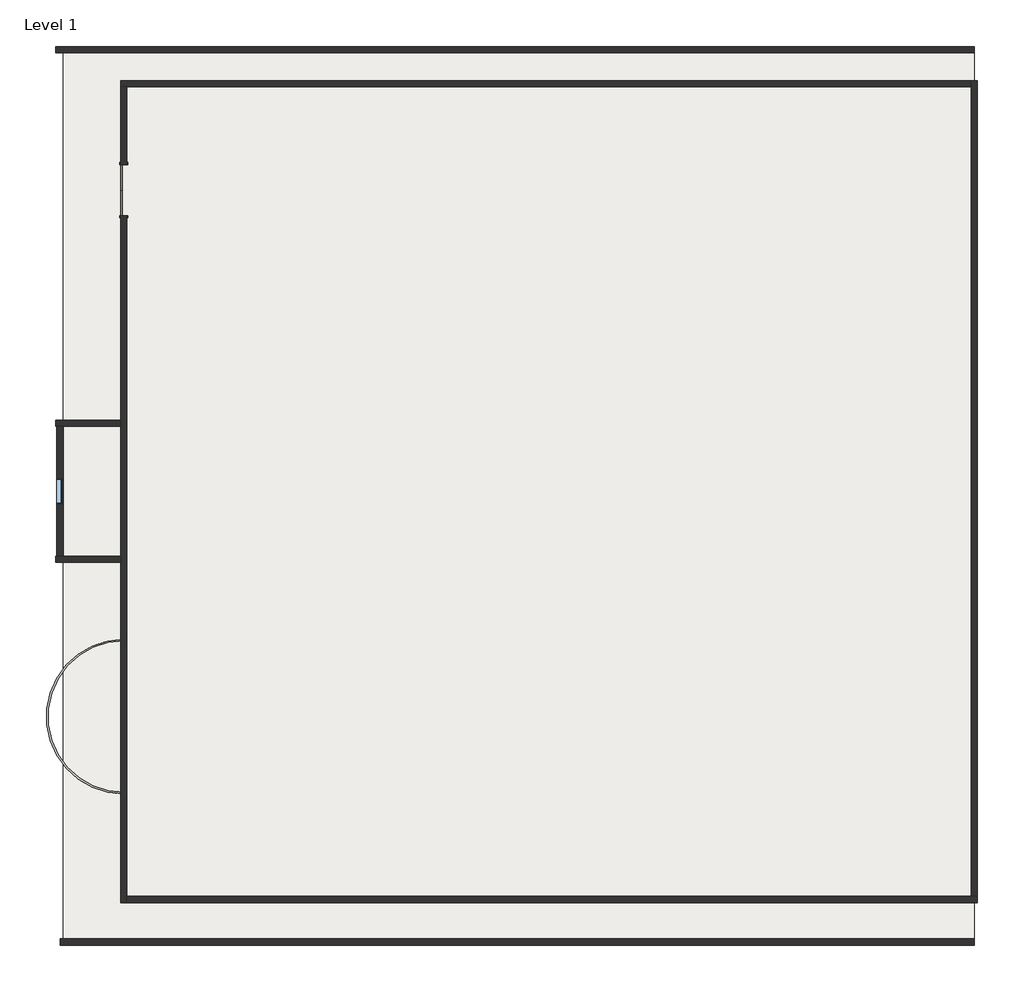
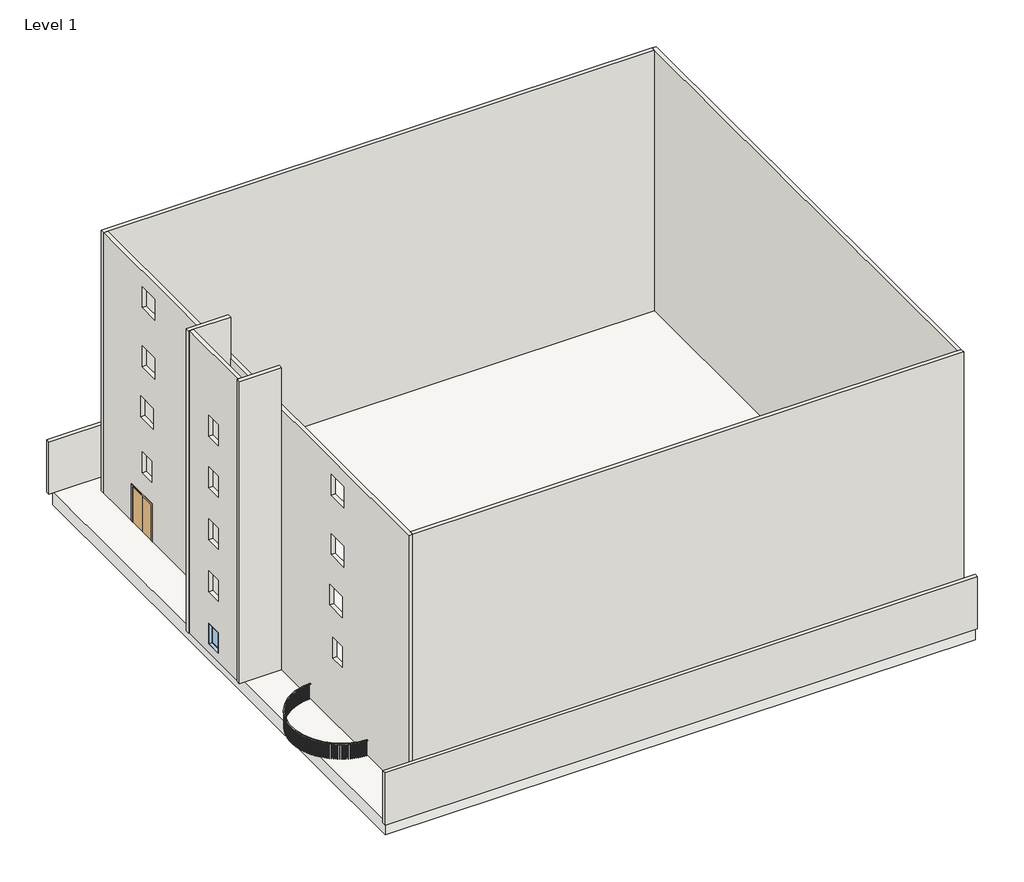
# One storey: 9 walls, 1 door, 1 railing, 1 slab, 1 window.
"""IFC4 building model written with IfcOpenShell, lengths in millimetres."""

from ifc_helpers import new_model, si_unit, point, frame, frame_2d, origin, origin_with_axes, place, context, project, spatial, polyline, circle_curve, trimmed, segment, composite_curve, outline, extrude, faceted_brep, transform, mapped, element, save
from components import door_640b4634, window_c1f32544

model = new_model("IFC4")

# Units and contexts
model_context = context("Model", 3, world=origin())
ifc_project = project(units=[si_unit("LENGTHUNIT", "METRE", prefix="MILLI")], contexts=[model_context])

# Site, building, storey
site = spatial("IfcSite", under=ifc_project)
building = spatial("IfcBuilding", under=site)
storey = spatial("IfcBuildingStorey", under=building, Name="Level 1", Elevation=0.0)

# Door
placement = place(None, origin())
door_shape = door_640b4634(model_context)
element("IfcDoor", 1, ObjectType="Door-Double-Flush_Panel : 72\" x 84\"", at=placement, inside=storey, context=model_context, shape_type="MappedRepresentation", body=[
    mapped(door_shape, transform((-15613.8723021, 10605.1556013, 0.0), x_axis=(0.0, 1.0, 0.0), y_axis=(-1.0, 0.0, 0.0), z_axis=(0.0, 0.0, 1.0))),
])

# Railing
element("IfcRailing", 2, ObjectType="Handrail - Rectangular", at=placement, inside=storey, context=model_context, shape_type="SweptSolid", body=[
    extrude(outline(composite_curve([segment(trimmed(circle_curve(frame_2d((-15613.8723021, -8267.0443987)), 2768.6), [point((-15613.8723021, -11035.6443987))], [point((-15613.8723021, -5498.4443987))], False, "CARTESIAN"), True, "CONTINUOUS"), segment(polyline([(-15613.8723021, -5498.4443987), (-15613.8723021, -5549.2443987)]), True, "CONTINUOUS"), segment(trimmed(circle_curve(frame_2d((-15613.8723021, -8267.0443987)), 2717.8), [point((-15613.8723021, -5549.2443987))], [point((-15613.8723021, -10984.8443987))], True, "CARTESIAN"), True, "CONTINUOUS"), segment(polyline([(-15613.8723021, -10984.8443987), (-15613.8723021, -11035.6443987)]), True, "CONTINUOUS")], self_intersect=False)), frame((0.0, 0.0, 863.6), z_axis=(0.0, 0.0, 1.0), x_axis=(1.0, 0.0, 0.0)), (0.0, 0.0, 1.0), 50.8),
    extrude(outline(polyline([(-15707.2871887, -11018.200394), (-15706.7066052, -10999.1592432), (-15687.6654545, -10999.7398266), (-15688.2460379, -11018.7809774), (-15707.2871887, -11018.200394)])), origin_with_axes(), (0.0, 0.0, 1.0), 863.6),
    extrude(outline(polyline([(-15809.094498, -11012.8546517), (-15807.8092461, -10993.8480574), (-15788.8026518, -10995.1333093), (-15790.0879037, -11014.1399036), (-15809.094498, -11012.8546517)])), origin_with_axes(), (0.0, 0.0, 1.0), 863.6),
    extrude(outline(polyline([(-15910.6340434, -11003.7427964), (-15908.6458859, -10984.7968277), (-15889.6999173, -10986.7849852), (-15891.6880747, -11005.7309539), (-15910.6340434, -11003.7427964)])), origin_with_axes(), (0.0, 0.0, 1.0), 863.6),
    extrude(outline(polyline([(-16011.7665548, -10990.8773258), (-16009.0782187, -10972.0179688), (-15990.2188616, -10974.7063049), (-15992.9071977, -10993.565662), (-16011.7665548, -10990.8773258)])), origin_with_axes(), (0.0, 0.0, 1.0), 863.6),
    extrude(outline(polyline([(-16112.3533203, -10974.275886), (-16108.9684927, -10955.5290078), (-16090.2216145, -10958.9138353), (-16093.6064421, -10977.6607135), (-16112.3533203, -10974.275886)])), origin_with_axes(), (0.0, 0.0, 1.0), 863.6),
    extrude(outline(polyline([(-16212.2563765, -10953.9612472), (-16208.1797001, -10935.3525608), (-16189.5710137, -10939.4292371), (-16193.6476901, -10958.0379235), (-16212.2563765, -10953.9612472)])), origin_with_axes(), (0.0, 0.0, 1.0), 863.6),
    extrude(outline(polyline([(-16311.3386979, -10929.9612727), (-16306.5757642, -10911.5163015), (-16288.130793, -10916.2792352), (-16292.8937267, -10934.7242064), (-16311.3386979, -10929.9612727)])), origin_with_axes(), (0.0, 0.0, 1.0), 863.6),
    extrude(outline(polyline([(-16409.4643846, -10902.3088806), (-16404.0217265, -10884.0529234), (-16385.7657693, -10889.4955816), (-16391.2084274, -10907.7515387), (-16409.4643846, -10902.3088806)])), origin_with_axes(), (0.0, 0.0, 1.0), 863.6),
    extrude(outline(polyline([(-16506.4988489, -10871.0419984), (-16500.3839313, -10853.0000949), (-16482.3420278, -10859.1150125), (-16488.4569454, -10877.156916), (-16506.4988489, -10871.0419984)])), origin_with_axes(), (0.0, 0.0, 1.0), 863.6),
    extrude(outline(polyline([(-16602.3089998, -10836.2035113), (-16595.5302099, -10818.4004074), (-16577.727106, -10825.1791974), (-16584.5058959, -10842.9823012), (-16602.3089998, -10836.2035113)])), origin_with_axes(), (0.0, 0.0, 1.0), 863.6),
    extrude(outline(polyline([(-16696.7634254, -10797.8412033), (-16689.3300608, -10780.3013176), (-16671.7901751, -10787.7346822), (-16679.2235397, -10805.2745679), (-16696.7634254, -10797.8412033)])), origin_with_axes(), (0.0, 0.0, 1.0), 863.6),
    extrude(outline(polyline([(-16789.7325734, -10756.0076916), (-16781.6548297, -10738.7550815), (-16764.4022196, -10746.8328252), (-16772.4799633, -10764.0854353), (-16789.7325734, -10756.0076916)])), origin_with_axes(), (0.0, 0.0, 1.0), 863.6),
    extrude(outline(polyline([(-16881.0889288, -10710.7603544), (-16872.3778853, -10693.8186833), (-16855.4362141, -10702.5297268), (-16864.1472577, -10719.471398), (-16881.0889288, -10710.7603544)])), origin_with_axes(), (0.0, 0.0, 1.0), 863.6),
    extrude(outline(polyline([(-16970.7071885, -10662.1612523), (-16961.374793, -10645.5537571), (-16944.7672979, -10654.8861526), (-16954.0996933, -10671.4936477), (-16970.7071885, -10662.1612523)])), origin_with_axes(), (0.0, 0.0, 1.0), 863.6),
    extrude(outline(polyline([(-17058.4644333, -10610.2770431), (-17048.5234862, -10594.0265025), (-17032.2729456, -10603.9674496), (-17042.2138927, -10620.2179902), (-17058.4644333, -10610.2770431)])), origin_with_axes(), (0.0, 0.0, 1.0), 863.6),
    extrude(outline(polyline([(-17144.2402968, -10555.1788904), (-17133.7044328, -10539.3075933), (-17117.8331358, -10549.8434573), (-17128.3689998, -10565.7147544), (-17144.2402968, -10555.1788904)])), origin_with_axes(), (0.0, 0.0, 1.0), 863.6),
    extrude(outline(polyline([(-17227.91713, -10496.942366), (-17216.8008, -10481.4720814), (-17201.3305154, -10492.5884114), (-17212.4468454, -10508.058696), (-17227.91713, -10496.942366)])), origin_with_axes(), (0.0, 0.0, 1.0), 863.6),
    extrude(outline(polyline([(-17309.3801631, -10435.6473464), (-17297.6986141, -10420.5992929), (-17282.6505606, -10432.2808419), (-17294.3321096, -10447.3288954), (-17309.3801631, -10435.6473464)])), origin_with_axes(), (0.0, 0.0, 1.0), 863.6),
    extrude(outline(polyline([(-17388.5176624, -10371.3779027), (-17376.2869166, -10356.7727202), (-17361.6817341, -10369.003466), (-17373.9124799, -10383.6086485), (-17388.5176624, -10371.3779027)])), origin_with_axes(), (0.0, 0.0, 1.0), 863.6),
    extrude(outline(polyline([(-17465.2210843, -10304.2221862), (-17452.4579172, -10290.0799068), (-17438.3156378, -10302.8430739), (-17451.0788049, -10316.9853533), (-17465.2210843, -10304.2221862)])), origin_with_axes(), (0.0, 0.0, 1.0), 863.6),
    extrude(outline(polyline([(-17539.3852234, -10234.2723065), (-17526.1071408, -10220.6123276), (-17512.4471619, -10233.8904102), (-17525.7252445, -10247.5503891), (-17539.3852234, -10234.2723065)])), origin_with_axes(), (0.0, 0.0, 1.0), 863.6),
    extrude(outline(polyline([(-17610.9083572, -10161.6242059), (-17597.1335711, -10148.4652634), (-17583.9746286, -10162.2400494), (-17597.7494146, -10175.398992), (-17610.9083572, -10161.6242059)])), origin_with_axes(), (0.0, 0.0, 1.0), 863.6),
    extrude(outline(polyline([(-17679.6923857, -10086.3775275), (-17665.4397894, -10073.7376699), (-17652.7999318, -10087.9902661), (-17667.052528, -10100.6301237), (-17679.6923857, -10086.3775275)])), origin_with_axes(), (0.0, 0.0, 1.0), 863.6),
    extrude(outline(polyline([(-17745.6429657, -10008.6354785), (-17730.9321079, -9996.5320424), (-17718.8286719, -10011.2429002), (-17733.5395296, -10023.3463362), (-17745.6429657, -10008.6354785)])), origin_with_axes(), (0.0, 0.0, 1.0), 863.6),
    extrude(outline(polyline([(-17808.6696403, -9928.5046887), (-17793.5206983, -9916.9542751), (-17781.9702847, -9932.1032172), (-17797.1192268, -9943.6536308), (-17808.6696403, -9928.5046887)])), origin_with_axes(), (0.0, 0.0, 1.0), 863.6),
    extrude(outline(polyline([(-17868.6859632, -9846.0950644), (-17853.1197149, -9835.1135157), (-17842.1381661, -9850.679764), (-17857.7044145, -9861.6613128), (-17868.6859632, -9846.0950644)])), origin_with_axes(), (0.0, 0.0, 1.0), 863.6),
    extrude(outline(polyline([(-17925.6096168, -9761.5196374), (-17909.6474126, -9751.1220157), (-17899.2497909, -9767.0842198), (-17915.2119951, -9777.4818416), (-17925.6096168, -9761.5196374)])), origin_with_axes(), (0.0, 0.0, 1.0), 863.6),
    extrude(outline(polyline([(-17979.3625254, -9674.8944101), (-17963.0262589, -9665.0949766), (-17953.2268254, -9681.4312431), (-17969.5630919, -9691.2306766), (-17979.3625254, -9674.8944101)])), origin_with_axes(), (0.0, 0.0, 1.0), 863.6),
    extrude(outline(polyline([(-18029.8709624, -9586.3381964), (-18013.1830402, -9577.1503918), (-18003.9952356, -9593.838314), (-18020.6831578, -9603.0261186), (-18029.8709624, -9586.3381964)])), origin_with_axes(), (0.0, 0.0, 1.0), 863.6),
    extrude(outline(polyline([(-18077.0656511, -9495.9724587), (-18060.0489621, -9487.408885), (-18051.4853883, -9504.425574), (-18068.5020774, -9512.9891477), (-18077.0656511, -9495.9724587)])), origin_with_axes(), (0.0, 0.0, 1.0), 863.6),
    extrude(outline(polyline([(-18120.88186, -9403.9211413), (-18103.559744, -9395.9935441), (-18095.6321467, -9413.3156601), (-18112.9542627, -9421.2432573), (-18120.88186, -9403.9211413)])), origin_with_axes(), (0.0, 0.0, 1.0), 863.6),
    extrude(outline(polyline([(-18161.2594914, -9310.3105005), (-18143.6557072, -9303.0297532), (-18136.3749598, -9320.6335374), (-18153.978744, -9327.9142847), (-18161.2594914, -9310.3105005)])), origin_with_axes(), (0.0, 0.0, 1.0), 863.6),
    extrude(outline(polyline([(-18198.1431639, -9215.2689313), (-18180.2818566, -9208.6450199), (-18173.6579452, -9226.5063272), (-18191.5192526, -9233.1302386), (-18198.1431639, -9215.2689313)])), origin_with_axes(), (0.0, 0.0, 1.0), 863.6),
    extrude(outline(polyline([(-18231.4822884, -9118.9267911), (-18213.3879563, -9112.9688011), (-18207.4299663, -9131.0631332), (-18225.5242984, -9137.0211233), (-18231.4822884, -9118.9267911)])), origin_with_axes(), (0.0, 0.0, 1.0), 863.6),
    extrude(outline(polyline([(-18261.2311376, -9021.4162217), (-18242.9285986, -9016.1323248), (-18237.6447018, -9034.4348638), (-18255.9472408, -9039.7187607), (-18261.2311376, -9021.4162217)])), origin_with_axes(), (0.0, 0.0, 1.0), 863.6),
    extrude(outline(polyline([(-18287.3489083, -8922.8709668), (-18268.8632659, -8918.2684105), (-18264.2607095, -8936.7540529), (-18282.7463519, -8941.3566093), (-18287.3489083, -8922.8709668)])), origin_with_axes(), (0.0, 0.0, 1.0), 863.6),
    extrude(outline(polyline([(-18309.7997777, -8823.4261899), (-18291.1563865, -8819.5112869), (-18287.2414835, -8838.1546781), (-18305.8848747, -8842.0695811), (-18309.7997777, -8823.4261899)])), origin_with_axes(), (0.0, 0.0, 1.0), 863.6),
    extrude(outline(polyline([(-18328.5529526, -8723.218288), (-18309.7773836, -8719.9964079), (-18306.5555035, -8738.7719768), (-18325.3310725, -8741.9938569), (-18328.5529526, -8723.218288)])), origin_with_axes(), (0.0, 0.0, 1.0), 863.6),
    extrude(outline(polyline([(-18343.5827113, -8622.3847046), (-18324.7007169, -8619.8602665), (-18322.1762788, -8638.7422609), (-18341.0582732, -8641.266699), (-18343.5827113, -8622.3847046)])), origin_with_axes(), (0.0, 0.0, 1.0), 863.6),
    extrude(outline(polyline([(-18354.8684394, -8521.0637416), (-18335.9059178, -8519.240208), (-18334.0823842, -8538.2027296), (-18353.0449058, -8540.0262632), (-18354.8684394, -8521.0637416)])), origin_with_axes(), (0.0, 0.0, 1.0), 863.6),
    extrude(outline(polyline([(-18362.3946574, -8419.3943695), (-18343.3776173, -8418.2742415), (-18342.2574894, -8437.2912816), (-18361.2745294, -8438.4114096), (-18362.3946574, -8419.3943695)])), origin_with_axes(), (0.0, 0.0, 1.0), 863.6),
    extrude(outline(polyline([(-18366.1510425, -8317.5160363), (-18347.1055675, -8317.1008504), (-18346.6903815, -8336.1463254), (-18365.7358565, -8336.5615114), (-18366.1510425, -8317.5160363)])), origin_with_axes(), (0.0, 0.0, 1.0), 863.6),
    extrude(outline(polyline([(-18366.1324425, -8215.5684771), (-18347.084655, -8215.8588025), (-18347.3749804, -8234.9065901), (-18366.422768, -8234.6162646), (-18366.1324425, -8215.5684771)])), origin_with_axes(), (0.0, 0.0, 1.0), 863.6),
    extrude(outline(polyline([(-18362.338883, -8113.6915214), (-18343.3149086, -8114.6869601), (-18344.3103473, -8133.7109345), (-18363.3343217, -8132.7154958), (-18362.338883, -8113.6915214)])), origin_with_axes(), (0.0, 0.0, 1.0), 863.6),
    extrude(outline(polyline([(-18354.775567, -8012.0249023), (-18335.8014988, -8013.7240889), (-18337.5006854, -8032.6981571), (-18356.4747536, -8030.9989705), (-18354.775567, -8012.0249023)])), origin_with_axes(), (0.0, 0.0, 1.0), 863.6),
    extrude(outline(polyline([(-18343.4528684, -7910.7080642), (-18324.5547309, -7913.1086681), (-18326.9553348, -7932.0068056), (-18345.8534723, -7929.6062017), (-18343.4528684, -7910.7080642)])), origin_with_axes(), (0.0, 0.0, 1.0), 863.6),
    extrude(outline(polyline([(-18328.3863172, -7809.8799718), (-18309.5900308, -7812.9787004), (-18312.6887594, -7831.7749867), (-18331.4850458, -7828.6762581), (-18328.3863172, -7809.8799718)])), origin_with_axes(), (0.0, 0.0, 1.0), 863.6),
    extrude(outline(polyline([(-18309.5965784, -7709.6789193), (-18290.9279238, -7713.4715225), (-18294.720527, -7732.140177), (-18313.3891815, -7728.3475739), (-18309.5965784, -7709.6789193)])), origin_with_axes(), (0.0, 0.0, 1.0), 863.6),
    extrude(outline(polyline([(-18287.1094237, -7610.2423412), (-18268.5940067, -7614.723617), (-18273.0752825, -7633.239034), (-18291.5906995, -7628.7577582), (-18287.1094237, -7610.2423412)])), origin_with_axes(), (0.0, 0.0, 1.0), 863.6),
    extrude(outline(polyline([(-18260.9556963, -7511.7066232), (-18242.6189123, -7516.8704251), (-18247.7827142, -7535.2072092), (-18266.1194983, -7530.0434072), (-18260.9556963, -7511.7066232)])), origin_with_axes(), (0.0, 0.0, 1.0), 863.6),
    extrude(outline(polyline([(-18231.1712682, -7414.2069153), (-18213.0382676, -7420.0461609), (-18218.8775132, -7438.1791615), (-18237.0105138, -7432.3399159), (-18231.1712682, -7414.2069153)])), origin_with_axes(), (0.0, 0.0, 1.0), 863.6),
    extrude(outline(polyline([(-18197.7969913, -7317.8769468), (-18179.8926451, -7324.383627), (-18186.3993252, -7342.2879732), (-18204.3036714, -7335.781293), (-18197.7969913, -7317.8769468)])), origin_with_axes(), (0.0, 0.0, 1.0), 863.6),
    extrude(outline(polyline([(-18160.8786412, -7222.8488425), (-18143.2275067, -7230.0140327), (-18150.392697, -7247.6651672), (-18168.0438315, -7240.499977), (-18160.8786412, -7222.8488425)])), origin_with_axes(), (0.0, 0.0, 1.0), 863.6),
    extrude(outline(polyline([(-18120.4668547, -7129.2529414), (-18103.0931419, -7137.0668141), (-18110.9070146, -7154.4405268), (-18128.2807273, -7146.6266541), (-18120.4668547, -7129.2529414)])), origin_with_axes(), (0.0, 0.0, 1.0), 863.6),
    extrude(outline(polyline([(-18076.6170598, -7037.2176184), (-18059.5445984, -7045.6694561), (-18067.9964361, -7062.7419175), (-18085.0688975, -7054.2900798), (-18076.6170598, -7037.2176184)])), origin_with_axes(), (0.0, 0.0, 1.0), 863.6),
    extrude(outline(polyline([(-18029.3894004, -6946.8691077), (-18012.6416066, -6955.9473181), (-18021.719817, -6972.6951119), (-18038.4676108, -6963.6169015), (-18029.3894004, -6946.8691077)])), origin_with_axes(), (0.0, 0.0, 1.0), 863.6),
    extrude(outline(polyline([(-17978.8486533, -6858.3313301), (-17962.4484981, -6868.0234615), (-17972.1406296, -6884.4236167), (-17988.5407847, -6874.7314853), (-17978.8486533, -6858.3313301)])), origin_with_axes(), (0.0, 0.0, 1.0), 863.6),
    extrude(outline(polyline([(-17925.0641393, -6771.7257227), (-17909.034117, -6782.0184816), (-17919.3268759, -6798.0485038), (-17935.3568982, -6787.7557449), (-17925.0641393, -6771.7257227)])), origin_with_axes(), (0.0, 0.0, 1.0), 863.6),
    extrude(outline(polyline([(-17868.1096285, -6687.1710723), (-17852.4717257, -6698.0503414), (-17863.3509947, -6713.6882442), (-17878.9888975, -6702.8089752), (-17868.1096285, -6687.1710723)])), origin_with_axes(), (0.0, 0.0, 1.0), 863.6),
    extrude(outline(polyline([(-17808.0632389, -6604.783353), (-17792.8389042, -6616.2342103), (-17804.2897615, -6631.458545), (-17819.5140962, -6620.0076878), (-17808.0632389, -6604.783353)])), origin_with_axes(), (0.0, 0.0, 1.0), 863.6),
    extrude(outline(polyline([(-17745.0073293, -6524.6755666), (-17730.2174442, -6536.6823063), (-17742.2241839, -6551.4721914), (-17757.014069, -6539.4654517), (-17745.0073293, -6524.6755666)])), origin_with_axes(), (0.0, 0.0, 1.0), 863.6),
    extrude(outline(polyline([(-17679.0283861, -6446.9575877), (-17664.6932362, -6459.5037415), (-17677.2393901, -6473.8388914), (-17691.57454, -6461.2927376), (-17679.0283861, -6446.9575877)])), origin_with_axes(), (0.0, 0.0, 1.0), 863.6),
    extrude(outline(polyline([(-17610.2169052, -6371.7360131), (-17596.3561524, -6384.804373), (-17609.4245123, -6398.6651258), (-17623.2852652, -6385.5967659), (-17610.2169052, -6371.7360131)])), origin_with_axes(), (0.0, 0.0, 1.0), 863.6),
    extrude(outline(polyline([(-17538.6672674, -6299.1140156), (-17525.2999229, -6312.6866572), (-17538.8725645, -6326.0540017), (-17552.239909, -6312.4813601), (-17538.6672674, -6299.1140156)])), origin_with_axes(), (0.0, 0.0, 1.0), 863.6),
    extrude(outline(polyline([(-17464.4776091, -6229.1912026), (-17451.6220073, -6243.2495098), (-17465.6803145, -6256.1051116), (-17478.5359163, -6242.0468044), (-17464.4776091, -6229.1912026)])), origin_with_axes(), (0.0, 0.0, 1.0), 863.6),
    extrude(outline(polyline([(-17387.7496877, -6162.063479), (-17375.4234611, -6176.5881697), (-17389.9481518, -6188.9143962), (-17402.2743784, -6174.3897055), (-17387.7496877, -6162.063479)])), origin_with_axes(), (0.0, 0.0, 1.0), 863.6),
    extrude(outline(polyline([(-17308.5887421, -6097.8229164), (-17296.8087973, -6112.7940687), (-17311.7799497, -6124.5740135), (-17323.5598944, -6109.6028612), (-17308.5887421, -6097.8229164)])), origin_with_axes(), (0.0, 0.0, 1.0), 863.6),
    extrude(outline(polyline([(-17227.1033483, -6036.5576261), (-17215.8858425, -6051.9547058), (-17231.2829223, -6063.1722116), (-17242.5004281, -6047.7751319), (-17227.1033483, -6036.5576261)])), origin_with_axes(), (0.0, 0.0, 1.0), 863.6),
    extrude(outline(polyline([(-17143.4052706, -5978.3516387), (-17132.7655895, -5994.1535274), (-17148.5674782, -6004.7932085), (-17159.2071593, -5988.9913198), (-17143.4052706, -5978.3516387)])), origin_with_axes(), (0.0, 0.0, 1.0), 863.6),
    extrude(outline(polyline([(-17057.6093079, -5923.2847887), (-17047.5620448, -5939.4698128), (-17063.7470688, -5949.5170759), (-17073.7943319, -5933.3320518), (-17057.6093079, -5923.2847887)])), origin_with_axes(), (0.0, 0.0, 1.0), 863.6),
    extrude(outline(polyline([(-16969.8331367, -5871.432605), (-16960.3920722, -5887.9785652), (-16976.9380325, -5897.4196297), (-16986.3790969, -5880.8736694), (-16969.8331367, -5871.432605)])), origin_with_axes(), (0.0, 0.0, 1.0), 863.6),
    extrude(outline(polyline([(-16880.1971495, -5822.8662071), (-16871.3752329, -5839.7504095), (-16888.2594352, -5848.5723261), (-16897.0813518, -5831.6881237), (-16880.1971495, -5822.8662071)])), origin_with_axes(), (0.0, 0.0, 1.0), 863.6),
    extrude(outline(polyline([(-16788.8242898, -5777.6522083), (-16780.6336211, -5794.8514945), (-16797.8329073, -5803.0421632), (-16806.023576, -5785.842877), (-16788.8242898, -5777.6522083)])), origin_with_axes(), (0.0, 0.0, 1.0), 863.6),
    extrude(outline(polyline([(-16695.8398832, -5735.8526231), (-16688.2916965, -5753.3434029), (-16705.7824763, -5760.8915896), (-16713.330663, -5743.4008098), (-16695.8398832, -5735.8526231)])), origin_with_axes(), (0.0, 0.0, 1.0), 863.6),
    extrude(outline(polyline([(-16601.3714657, -5697.5247835), (-16594.4761141, -5715.2830668), (-16612.2343974, -5722.1784184), (-16619.129749, -5704.4201351), (-16601.3714657, -5697.5247835)])), origin_with_axes(), (0.0, 0.0, 1.0), 863.6),
    extrude(outline(polyline([(-16505.5486089, -5662.7212592), (-16499.3155499, -5680.722689), (-16517.3169798, -5686.955748), (-16523.5500387, -5668.9543181), (-16505.5486089, -5662.7212592)])), origin_with_axes(), (0.0, 0.0, 1.0), 863.6),
    extrude(outline(polyline([(-16408.502742, -5631.4897862), (-16402.9405248, -5649.7096721), (-16421.1604106, -5655.2718893), (-16426.7226278, -5637.0520034), (-16408.502742, -5631.4897862)])), origin_with_axes(), (0.0, 0.0, 1.0), 863.6),
    extrude(outline(polyline([(-16310.3669716, -5603.8732013), (-16305.4832253, -5622.286553), (-16323.896577, -5627.1702994), (-16328.7803233, -5608.7569477), (-16310.3669716, -5603.8732013)])), origin_with_axes(), (0.0, 0.0, 1.0), 863.6),
    extrude(outline(polyline([(-16211.2758994, -5579.9093829), (-16207.0773224, -5598.490945), (-16225.6588845, -5602.689522), (-16229.8574615, -5584.1079599), (-16211.2758994, -5579.9093829)])), origin_with_axes(), (0.0, 0.0, 1.0), 863.6),
    extrude(outline(polyline([(-16111.3654371, -5559.6311994), (-16107.8577882, -5578.3554857), (-16126.5820745, -5581.8631347), (-16130.0897235, -5563.1388484), (-16111.3654371, -5559.6311994)])), origin_with_axes(), (0.0, 0.0, 1.0), 863.6),
    extrude(outline(polyline([(-16010.7726206, -5543.0664641), (-16007.9607107, -5561.9077926), (-16026.8020393, -5564.7197026), (-16029.6139492, -5545.878374), (-16010.7726206, -5543.0664641)])), origin_with_axes(), (0.0, 0.0, 1.0), 863.6),
    extrude(outline(polyline([(-15909.6354215, -5530.2378969), (-15907.5231074, -5549.1704252), (-15926.4556357, -5551.2827393), (-15928.5679498, -5532.3502109), (-15909.6354215, -5530.2378969)])), origin_with_axes(), (0.0, 0.0, 1.0), 863.6),
    extrude(outline(polyline([(-15808.092558, -5521.1630933), (-15806.682737, -5540.1608538), (-15825.6804975, -5541.5706748), (-15827.0903185, -5522.5729143), (-15808.092558, -5521.1630933)])), origin_with_axes(), (0.0, 0.0, 1.0), 863.6),
    extrude(outline(polyline([(-15706.2833048, -5515.8545002), (-15705.5779106, -5534.8914358), (-15724.6148462, -5535.5968301), (-15725.3202405, -5516.5598944), (-15706.2833048, -5515.8545002)])), origin_with_axes(), (0.0, 0.0, 1.0), 863.6),
    extrude(outline(polyline([(-15632.9552984, -11019.719732), (-15632.8891527, -11000.6698468), (-15613.8392675, -11000.7359925), (-15613.9054132, -11019.7858777), (-15632.9552984, -11019.719732)])), origin_with_axes(), (0.0, 0.0, 1.0), 863.6),
    extrude(outline(polyline([(-15613.9054132, -5514.3029197), (-15613.8392675, -5533.3528049), (-15632.8891527, -5533.4189506), (-15632.9552984, -5514.3690654), (-15613.9054132, -5514.3029197)])), origin_with_axes(), (0.0, 0.0, 1.0), 863.6),
])

# Slab
element("IfcSlab", 3, ObjectType="Generic - 12\"", at=placement, inside=storey, context=model_context, shape_type="SweptSolid", body=[
    extrude(outline(polyline([(14866.1276979, 15634.3556013), (14866.1276979, -16229.9443987), (-17785.5723021, -16229.9443987), (-17785.5723021, 15634.3556013), (14866.1276979, 15634.3556013)])), frame((0.0, 0.0, -762.0), z_axis=(0.0, 0.0, 1.0), x_axis=(1.0, 0.0, 0.0)), (0.0, 0.0, 1.0), 762.0),
])

# Walls
element("IfcWall", 4, at=placement, inside=storey, context=model_context, shape_type="SweptSolid", body=[
    extrude(outline(polyline([(2134.2556013, 0.0), (-2513.9443987, 0.0), (-2513.9443987, 17678.4), (2134.2556013, 17678.4), (2134.2556013, 0.0)]), holes=[polyline([(-647.0443987, 13868.7091362), (-647.0443987, 12649.5091362), (267.3556013, 12649.5091362), (267.3556013, 13868.7091362), (-647.0443987, 13868.7091362)]), polyline([(-647.0443987, 10854.6470019), (-647.0443987, 9635.4470019), (267.3556013, 9635.4470019), (267.3556013, 10854.6470019), (-647.0443987, 10854.6470019)]), polyline([(-647.0443987, 7811.9274554), (-647.0443987, 6592.7274554), (267.3556013, 6592.7274554), (267.3556013, 7811.9274554), (-647.0443987, 7811.9274554)]), polyline([(-647.0443987, 4760.964574), (-647.0443987, 3541.764574), (267.3556013, 3541.764574), (267.3556013, 4760.964574), (-647.0443987, 4760.964574)]), polyline([(-647.0443987, 1708.9712758), (-647.0443987, 489.7712758), (267.3556013, 489.7712758), (267.3556013, 1708.9712758), (-647.0443987, 1708.9712758)])]), frame((-18014.1723021, 0.0, 0.0), z_axis=(1.0, 0.0, 0.0), x_axis=(0.0, 1.0, 0.0)), (0.0, 0.0, 1.0), 228.6),
])
element("IfcWall", 5, ObjectType="Generic - 8\"", at=placement, inside=storey, context=model_context, shape_type="Brep", body=[
    faceted_brep([(-15728.1723021, 14300.8556013, 0.0), (-15499.5723021, 14300.8556013, 0.0), (14751.8276979, 14300.8556013, 0.0), (14751.8276979, 14300.8556013, 15240.0), (-15499.5723021, 14300.8556013, 15240.0), (-15728.1723021, 14300.8556013, 15240.0), (-15728.1723021, 14529.4556013, 0.0), (-15728.1723021, 14529.4556013, 15240.0), (14751.8276979, 14529.4556013, 15240.0), (14751.8276979, 14529.4556013, 0.0)], [[[0, 1, 2, 3, 4, 5]], [[6, 7, 8, 9]], [[2, 1, 0, 6, 9]], [[5, 4, 3, 8, 7]], [[0, 5, 7, 6]], [[3, 2, 9, 8]]]),
])
element("IfcWall", 6, ObjectType="Generic - 8\"", at=placement, inside=storey, context=model_context, shape_type="Brep", body=[
    faceted_brep([(-15499.5723021, 14300.8556013, 15240.0), (-15499.5723021, -14705.9443987, 15240.0), (-15499.5723021, -14934.5443987, 15240.0), (-15499.5723021, -14934.5443987, 0.0), (-15499.5723021, -14705.9443987, 0.0), (-15499.5723021, 9690.7556013, 0.0), (-15499.5723021, 9690.7556013, 2133.6), (-15499.5723021, 11519.5556013, 2133.6), (-15499.5723021, 11519.5556013, 0.0), (-15499.5723021, 14300.8556013, 0.0), (-15499.5723021, 9690.7556013, 4652.5653391), (-15499.5723021, 10605.1556013, 4652.5653391), (-15499.5723021, 10605.1556013, 3433.3653391), (-15499.5723021, 9690.7556013, 3433.3653391), (-15499.5723021, -7657.4443987, 4891.3089798), (-15499.5723021, -7657.4443987, 3672.1089798), (-15499.5723021, -8571.8443987, 3672.1089798), (-15499.5723021, -8571.8443987, 4891.3089798), (-15499.5723021, 10757.5556013, 7835.3919963), (-15499.5723021, 10757.5556013, 6616.1919963), (-15499.5723021, 9538.3556013, 6616.1919963), (-15499.5723021, 9538.3556013, 7835.3919963), (-15499.5723021, 10605.1556013, 10870.7054136), (-15499.5723021, 10605.1556013, 9651.5054136), (-15499.5723021, 9385.9556013, 9651.5054136), (-15499.5723021, 9385.9556013, 10870.7054136), (-15499.5723021, 10605.1556013, 14325.6), (-15499.5723021, 10605.1556013, 13106.4), (-15499.5723021, 9385.9556013, 13106.4), (-15499.5723021, 9385.9556013, 14325.6), (-15499.5723021, -7352.6443987, 7813.3755614), (-15499.5723021, -7352.6443987, 6594.1755614), (-15499.5723021, -8571.8443987, 6594.1755614), (-15499.5723021, -8571.8443987, 7813.3755614), (-15499.5723021, -7505.0443987, 10858.7499872), (-15499.5723021, -7505.0443987, 9639.5499872), (-15499.5723021, -8724.2443987, 9639.5499872), (-15499.5723021, -8724.2443987, 10858.7499872), (-15499.5723021, -7505.0443987, 14325.6), (-15499.5723021, -7505.0443987, 13106.4), (-15499.5723021, -8724.2443987, 13106.4), (-15499.5723021, -8724.2443987, 14325.6), (-15499.5723021, -37.4443987, 7662.6452052), (-15499.5723021, 876.9556013, 7662.6452052), (-15499.5723021, 876.9556013, 5833.8452052), (-15499.5723021, -37.4443987, 5833.8452052), (-15728.1723021, -14934.5443987, 15240.0), (-15728.1723021, 14300.8556013, 15240.0), (-15728.1723021, 14300.8556013, 0.0), (-15728.1723021, 11519.5556013, 0.0), (-15728.1723021, 11519.5556013, 2133.6), (-15728.1723021, 9690.7556013, 2133.6), (-15728.1723021, 9690.7556013, 0.0), (-15728.1723021, 2362.8556013, 0.0), (-15728.1723021, 2134.2556013, 0.0), (-15728.1723021, -2513.9443987, 0.0), (-15728.1723021, -2742.5443987, 0.0), (-15728.1723021, -14934.5443987, 0.0), (-15728.1723021, 9690.7556013, 4652.5653391), (-15728.1723021, 9690.7556013, 3433.3653391), (-15728.1723021, 10605.1556013, 3433.3653391), (-15728.1723021, 10605.1556013, 4652.5653391), (-15728.1723021, -7657.4443987, 4891.3089798), (-15728.1723021, -8571.8443987, 4891.3089798), (-15728.1723021, -8571.8443987, 3672.1089798), (-15728.1723021, -7657.4443987, 3672.1089798), (-15728.1723021, 10757.5556013, 7835.3919963), (-15728.1723021, 9538.3556013, 7835.3919963), (-15728.1723021, 9538.3556013, 6616.1919963), (-15728.1723021, 10757.5556013, 6616.1919963), (-15728.1723021, 10605.1556013, 10870.7054136), (-15728.1723021, 9385.9556013, 10870.7054136), (-15728.1723021, 9385.9556013, 9651.5054136), (-15728.1723021, 10605.1556013, 9651.5054136), (-15728.1723021, 10605.1556013, 14325.6), (-15728.1723021, 9385.9556013, 14325.6), (-15728.1723021, 9385.9556013, 13106.4), (-15728.1723021, 10605.1556013, 13106.4), (-15728.1723021, -7352.6443987, 7813.3755614), (-15728.1723021, -8571.8443987, 7813.3755614), (-15728.1723021, -8571.8443987, 6594.1755614), (-15728.1723021, -7352.6443987, 6594.1755614), (-15728.1723021, -7505.0443987, 10858.7499872), (-15728.1723021, -8724.2443987, 10858.7499872), (-15728.1723021, -8724.2443987, 9639.5499872), (-15728.1723021, -7505.0443987, 9639.5499872), (-15728.1723021, -7505.0443987, 14325.6), (-15728.1723021, -8724.2443987, 14325.6), (-15728.1723021, -8724.2443987, 13106.4), (-15728.1723021, -7505.0443987, 13106.4), (-15728.1723021, -37.4443987, 7662.6452052), (-15728.1723021, -37.4443987, 5833.8452052), (-15728.1723021, 876.9556013, 5833.8452052), (-15728.1723021, 876.9556013, 7662.6452052)], [[[0, 1, 2, 3, 4, 5, 6, 7, 8, 9], [10, 11, 12, 13], [14, 15, 16, 17], [18, 19, 20, 21], [22, 23, 24, 25], [26, 27, 28, 29], [30, 31, 32, 33], [34, 35, 36, 37], [38, 39, 40, 41], [42, 43, 44, 45]], [[46, 47, 48, 49, 50, 51, 52, 53, 54, 55, 56, 57], [58, 59, 60, 61], [62, 63, 64, 65], [66, 67, 68, 69], [70, 71, 72, 73], [74, 75, 76, 77], [78, 79, 80, 81], [82, 83, 84, 85], [86, 87, 88, 89], [90, 91, 92, 93]], [[3, 57, 56, 55, 54, 53, 52, 5, 4]], [[48, 9, 8, 49]], [[2, 1, 0, 47, 46]], [[3, 2, 46, 57]], [[0, 9, 48, 47]], [[7, 50, 49, 8]], [[50, 7, 6, 51]], [[51, 6, 5, 52]], [[59, 58, 10, 13]], [[60, 59, 13, 12]], [[61, 60, 12, 11]], [[58, 61, 11, 10]], [[15, 14, 62, 65]], [[16, 15, 65, 64]], [[17, 16, 64, 63]], [[14, 17, 63, 62]], [[19, 18, 66, 69]], [[20, 19, 69, 68]], [[21, 20, 68, 67]], [[18, 21, 67, 66]], [[23, 22, 70, 73]], [[24, 23, 73, 72]], [[25, 24, 72, 71]], [[22, 25, 71, 70]], [[27, 26, 74, 77]], [[28, 27, 77, 76]], [[29, 28, 76, 75]], [[26, 29, 75, 74]], [[31, 30, 78, 81]], [[32, 31, 81, 80]], [[33, 32, 80, 79]], [[30, 33, 79, 78]], [[35, 34, 82, 85]], [[36, 35, 85, 84]], [[37, 36, 84, 83]], [[34, 37, 83, 82]], [[39, 38, 86, 89]], [[40, 39, 89, 88]], [[41, 40, 88, 87]], [[38, 41, 87, 86]], [[91, 90, 42, 45]], [[92, 91, 45, 44]], [[93, 92, 44, 43]], [[90, 93, 43, 42]]]),
])
element("IfcWall", 7, ObjectType="Generic - 8\"", at=placement, inside=storey, context=model_context, shape_type="Brep", body=[
    faceted_brep([(14980.4276979, -14705.9443987, 0.0), (14751.8276979, -14705.9443987, 0.0), (-15499.5723021, -14705.9443987, 0.0), (-15499.5723021, -14705.9443987, 15240.0), (14751.8276979, -14705.9443987, 15240.0), (14980.4276979, -14705.9443987, 15240.0), (14980.4276979, -14934.5443987, 0.0), (14980.4276979, -14934.5443987, 15240.0), (-15499.5723021, -14934.5443987, 15240.0), (-15499.5723021, -14934.5443987, 0.0)], [[[0, 1, 2, 3, 4, 5]], [[6, 7, 8, 9]], [[2, 1, 0, 6, 9]], [[5, 4, 3, 8, 7]], [[0, 5, 7, 6]], [[3, 2, 9, 8]]]),
])
element("IfcWall", 8, ObjectType="Generic - 8\"", at=placement, inside=storey, context=model_context, shape_type="Brep", body=[
    faceted_brep([(14751.8276979, 14529.4556013, 0.0), (14751.8276979, 14300.8556013, 0.0), (14751.8276979, -14705.9443987, 0.0), (14751.8276979, -14705.9443987, 15240.0), (14751.8276979, 14300.8556013, 15240.0), (14751.8276979, 14529.4556013, 15240.0), (14980.4276979, 14529.4556013, 0.0), (14980.4276979, 14529.4556013, 15240.0), (14980.4276979, -14705.9443987, 15240.0), (14980.4276979, -14705.9443987, 0.0)], [[[0, 1, 2, 3, 4, 5]], [[6, 7, 8, 9]], [[2, 1, 0, 6, 9]], [[5, 4, 3, 8, 7]], [[0, 5, 7, 6]], [[3, 2, 9, 8]]]),
])
element("IfcWall", 9, ObjectType="Generic - 8\"", at=placement, inside=storey, context=model_context, shape_type="Brep", body=[
    faceted_brep([(-18052.2723021, 2134.2556013, 0.0), (-18014.1723021, 2134.2556013, 0.0), (-17785.5723021, 2134.2556013, 0.0), (-15728.1723021, 2134.2556013, 0.0), (-15728.1723021, 2134.2556013, 17678.4), (-17785.5723021, 2134.2556013, 17678.4), (-18014.1723021, 2134.2556013, 17678.4), (-18052.2723021, 2134.2556013, 17678.4), (-18052.2723021, 2362.8556013, 0.0), (-18052.2723021, 2362.8556013, 17678.4), (-15728.1723021, 2362.8556013, 17678.4), (-15728.1723021, 2362.8556013, 0.0)], [[[0, 1, 2, 3, 4, 5, 6, 7]], [[8, 9, 10, 11]], [[3, 2, 1, 0, 8, 11]], [[7, 6, 5, 4, 10, 9]], [[0, 7, 9, 8]], [[4, 3, 11, 10]]]),
])
element("IfcWall", 10, ObjectType="Generic - 8\"", at=placement, inside=storey, context=model_context, shape_type="Brep", body=[
    faceted_brep([(-18052.2723021, -2742.5443987, 0.0), (-15728.1723021, -2742.5443987, 0.0), (-15728.1723021, -2742.5443987, 17678.4), (-18052.2723021, -2742.5443987, 17678.4), (-18052.2723021, -2513.9443987, 0.0), (-18052.2723021, -2513.9443987, 17678.4), (-18014.1723021, -2513.9443987, 17678.4), (-17785.5723021, -2513.9443987, 17678.4), (-15728.1723021, -2513.9443987, 17678.4), (-15728.1723021, -2513.9443987, 0.0), (-17785.5723021, -2513.9443987, 0.0), (-18014.1723021, -2513.9443987, 0.0)], [[[0, 1, 2, 3]], [[4, 5, 6, 7, 8, 9, 10, 11]], [[1, 0, 4, 11, 10, 9]], [[3, 2, 8, 7, 6, 5]], [[0, 3, 5, 4]], [[2, 1, 9, 8]]]),
])
element("IfcWall", 11, ObjectType="Generic - 8\"", at=placement, inside=storey, context=model_context, shape_type="SweptSolid", body=[
    extrude(outline(polyline([(14866.1276979, 15520.0556013), (-18052.2723021, 15520.0556013), (-18052.2723021, 15748.6556013), (14866.1276979, 15748.6556013), (14866.1276979, 15520.0556013)])), origin_with_axes(), (0.0, 0.0, 1.0), 3048.0),
])
element("IfcWall", 12, ObjectType="Generic - 8\"", at=placement, inside=storey, context=model_context, shape_type="SweptSolid", body=[
    extrude(outline(polyline([(14866.1276979, -16458.5443987), (-17899.8723021, -16458.5443987), (-17899.8723021, -16229.9443987), (14866.1276979, -16229.9443987), (14866.1276979, -16458.5443987)])), origin_with_axes(), (0.0, 0.0, 1.0), 3048.0),
])

# Window
window_shape = window_c1f32544(model_context)
element("IfcWindow", 13, ObjectType="Fixed : 36\" x 48\"", at=placement, inside=storey, context=model_context, shape_type="MappedRepresentation", body=[
    mapped(window_shape, transform((-17899.8723021, -227.9443987, -424.6287242), x_axis=(0.0, -1.0, 0.0), y_axis=(1.0, 0.0, 0.0), z_axis=(0.0, 0.0, 1.0))),
])

save(model, "model.ifc")

# Revit data of these elements
# Type "Door-Double-Flush_Panel : 72\" x 84\""
#   Type Mark = "8"
#   Construction Type Id = "DOOR"
#   Assembly Code = "C1020"
#   Analytic Construction = "Wooden"
#   Thickness = 0' - 2"
#   Thermal Resistance (R) = 2.5876 (h·ft²·°F)/BTU
#   Swing Angle [instance default] = 90.00°
#   Panel Width = 3' - 0"
#   Heat Transfer Coefficient (U) = 0.3865 BTU/(h·ft²·°F)
#   Height = 7' - 0"
#   Trim Projection Ext = 0' - 1"
#   Trim Projection Int = 0' - 1"
#   Trim Width = 0' - 3"
#   Width = 6' - 0"
#   Define Thermal Properties by = 1
#   Panel Material = Wood - Birch - Solid Stained Light Low Gloss
#   Trim Material = Paint - Sienna
#   Visual Light Transmittance = 0
#   Solar Heat Gain Coefficient = 0
#   Function = (empty or 0)
#   Wall Closure = (empty or 0)
# Type "Handrail - Rectangular"
#   Assembly Code = "C2010400"
#   built-in parameter 1008612 = 0.0416667 (stored number, unit not read)
#   built-in parameter 1008611 = 0.0416667 (stored number, unit not read)
#   built-in parameter 1008609 = 0.333333 (stored number, unit not read)
#   built-in parameter 1008604 = 0.166667 (stored number, unit not read)
#   built-in parameter 1008603 = 0.166667 (stored number, unit not read)
#   Railing Height = 3' - 0"
#   built-in parameter 1008630 = 2
#   built-in parameter 1008610 = 2
#   built-in parameter 1008618 = Baluster - Square : 3/4"
# Type "Generic - 12\""
#   Assembly Code = "B1010"
#   Function = 0
#   Layers, outside or top first: 2' - 6" no material (function 1)
# Type
#   Assembly Code = "B2010"
#   Layers, outside or top first: 0' - 9" "Acoustic Ceiling Tile 24 x 24" (function 1)
# Type "Generic - 8\""
#   Assembly Code = "B2010"
#   Layers, outside or top first: 0' - 9" "Acoustic Ceiling Tile 24 x 24" (function 1)
# Type "Fixed : 36\" x 48\""
#   Type Mark = "1"
#   Construction Type Id = "GSP4R"
#   Assembly Code = "B2020100"
#   Analytic Construction = "1/8 in Pilkington single glazing"
#   Visual Light Transmittance = 0.9
#   Solar Heat Gain Coefficient = 0.78
#   Heat Transfer Coefficient (U) = 0.6496 BTU/(h·ft²·°F)
#   Height = 4' - 0"
#   Default Sill Height = 3' - 0"
#   Width = 3' - 0"
#   Window Inset = 0' - 0 3/4"
#   Define Thermal Properties by = 1
#   Glass Pane Material = Glass
#   Sash Material = Sash
#   Wall Closure = (empty or 0)
# Element 1 (IfcDoor, "Door-Double-Flush_Panel : 72\" x 84\"")
#   Swing Angle = 90.00°
#   Phase Created = New Construction
#   Materials on its faces: "Paint - Sienna", "Wood - Birch - Solid Stained Light Low Gloss"
# Element 2 (IfcRailing, "Handrail - Rectangular")
#   Phase Created = New Construction
# Element 3 (IfcSlab, "Generic - 12\"")
#   Height Offset From Level = 0' - 0"
#   Phase Created = New Construction
#   Materials on its faces: "Default Floor"
# Element 4 (IfcWall)
#   Top Offset = 0' - 0"
#   Base Offset = 0' - 0"
#   Unconnected Height = 58' - 0"
#   wall height = 58' - 0"
#   Phase Created = New Construction
#   Base Constraint = Level 1
#   Materials on its faces: "Acoustic Ceiling Tile 24 x 24"
# Elements 5, 6, 7, 8 (IfcWall, "Generic - 8\"")
#   Top Offset = 0' - 0"
#   Base Offset = 0' - 0"
#   Unconnected Height = 50' - 0"
#   wall height = 50' - 0"
#   Phase Created = New Construction
#   Base Constraint = Level 1
#   Materials on its faces: "Acoustic Ceiling Tile 24 x 24"
# Elements 9, 10 (IfcWall, "Generic - 8\"")
#   Top Offset = 0' - 0"
#   Base Offset = 0' - 0"
#   Unconnected Height = 58' - 0"
#   wall height = 58' - 0"
#   Phase Created = New Construction
#   Base Constraint = Level 1
#   Materials on its faces: "Acoustic Ceiling Tile 24 x 24"
# Elements 11, 12 (IfcWall, "Generic - 8\"")
#   Top Offset = 0' - 0"
#   Base Offset = 0' - 0"
#   Unconnected Height = 10' - 0"
#   wall height = 10' - 0"
#   Phase Created = New Construction
#   Base Constraint = Level 1
#   Materials on its faces: "Acoustic Ceiling Tile 24 x 24"
# Element 13 (IfcWindow, "Fixed : 36\" x 48\"")
#   Mark = "24"
#   Phase Created = New Construction
#   Materials on its faces: "Sash", "Glass"
# Materials
#   "Wood - Birch - Solid Stained Light Low Gloss": class "Wood", colour RGB 210 159 95, transparency 0, Cost = 0
#   "Paint - Sienna": colour RGB 118 70 51, transparency 0, Cost = 0
#   "Acoustic Ceiling Tile 24 x 24": class "Generic", colour RGB 232 232 232, transparency 0, Description = "Acoustic Ceiling Tile 24 x 24", Cost = 0
#   "Glass": class "Glass", colour RGB 0 128 192, transparency 0.75, Description = "Soda Lime Glass", Cost = 0
#   "Sash": class "Wood", colour RGB 224 178 126, transparency 0
#   "Default Floor": colour RGB 128 128 128, transparency 0
